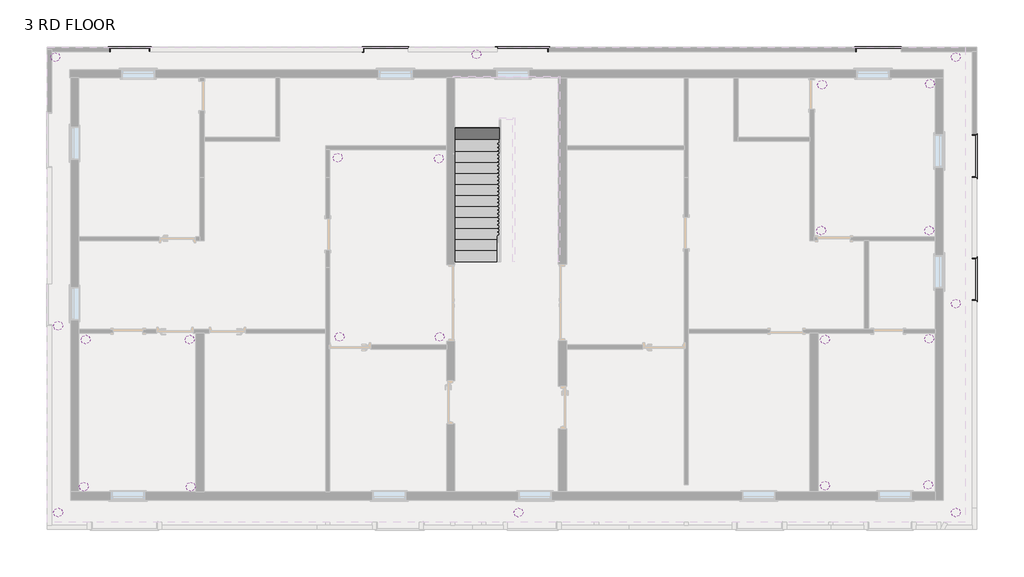
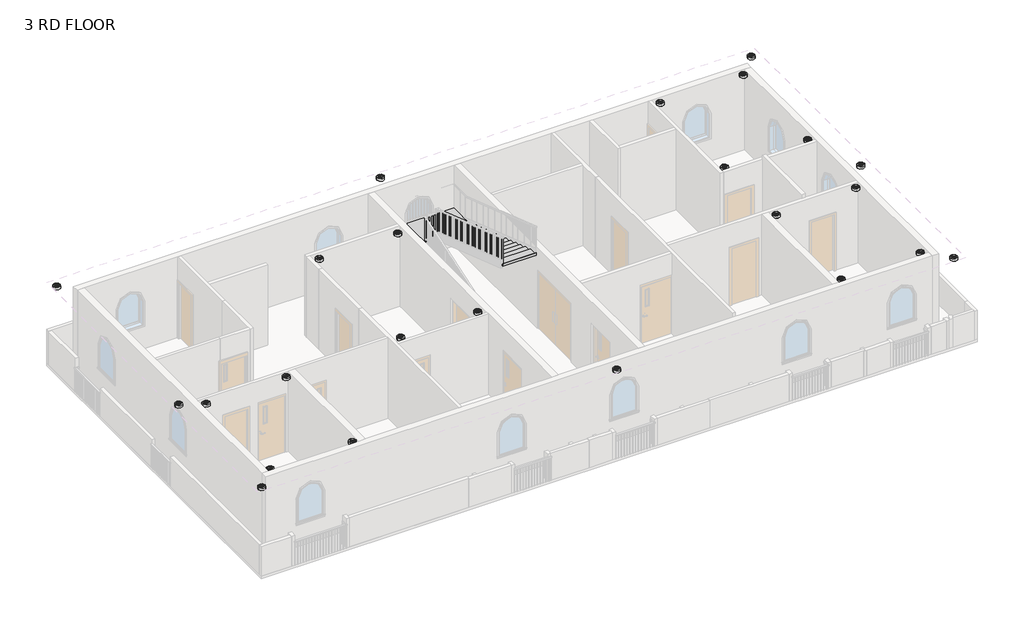
# One storey, part 6 of 7: 24 light fixtures, 6 railings, 1 stair flight.
# Revit data of these elements (continued)
# Element 21 (IfcLightFixture, "Ceiling Light - Flat Round : 60W - 120V") (continued)
#   Phase Created = New Construction
#   Materials on its faces: "Glass, White, High Luminance", "Steel, Paint Finish, Dark Gray, Matte"
# Element 22 (IfcLightFixture, "Ceiling Light - Flat Round : 60W - 120V")
#   Mark = "109"
#   built-in parameter 1140040 = 1
#   Phase Created = New Construction
#   Materials on its faces: "Glass, White, High Luminance", "Steel, Paint Finish, Dark Gray, Matte"
# Element 23 (IfcLightFixture, "Ceiling Light - Flat Round : 60W - 120V")
#   Mark = "110"
#   built-in parameter 1140040 = 1
#   Phase Created = New Construction
#   Materials on its faces: "Glass, White, High Luminance", "Steel, Paint Finish, Dark Gray, Matte"
# Element 24 (IfcLightFixture, "Ceiling Light - Flat Round : 60W - 120V")
#   Mark = "111"
#   built-in parameter 1140040 = 1
#   Phase Created = New Construction
#   Materials on its faces: "Glass, White, High Luminance", "Steel, Paint Finish, Dark Gray, Matte"
# Elements 25, 26, 27, 28, 29, 30 (IfcRailing, "Handrail - Rectangular")
#   Phase Created = New Construction
# Element 31 (IfcStairFlight, "2\" Tread 1\" Nosing 1/4\" Riser")
#   Phase Created = New Construction
# Materials
#   "Steel, Paint Finish, Dark Gray, Matte": class "Metal", colour RGB 98 98 98, transparency 0, Description = "Steel, paint finish, dark gray, matte", Cost = 0
#   "Glass, White, High Luminance": class "Glass", colour RGB 249 250 249, transparency 0.8, Description = "physical material", Cost = 0
